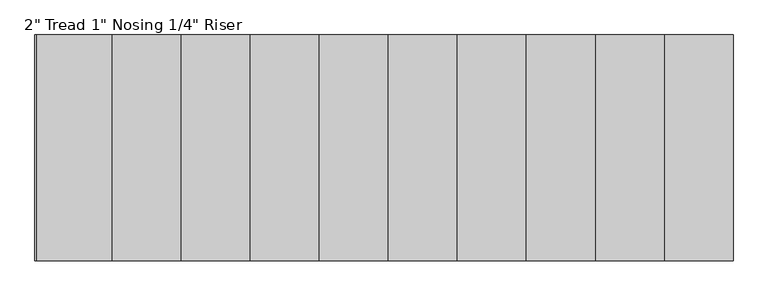
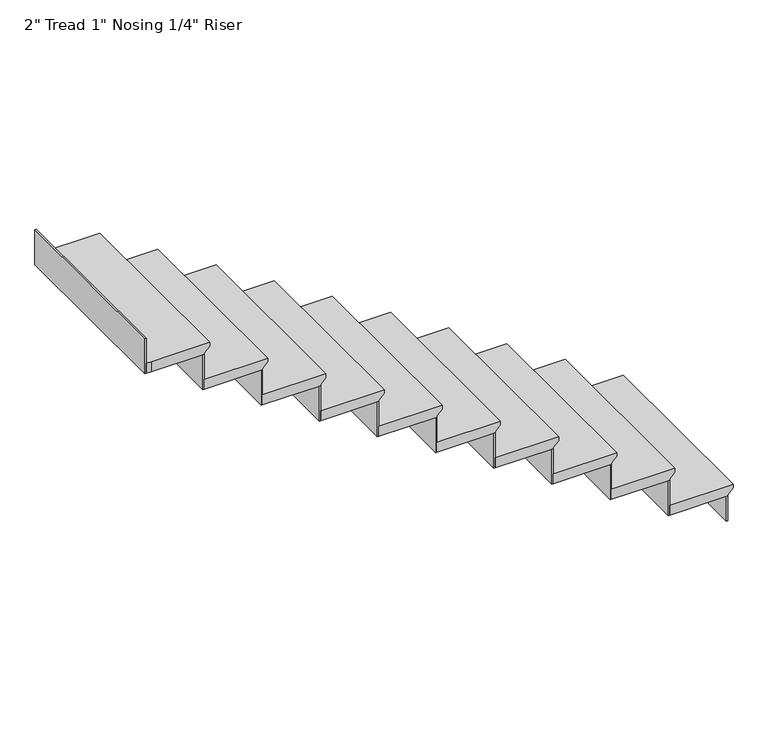
"""IFC4 building model written with IfcOpenShell, lengths in millimetres: stair flight geometry."""

from ifc_helpers import new_model, si_unit, origin, place, context, project, spatial, faceted_brep, source, transform, mapped, element, save


def stair_flight_b5a9fedd(model_context):
    return source(origin(), model_context, "Body", "Brep", [
        faceted_brep([(13347.9752377, 21801.2384539, 158.75), (13347.9752377, 21801.2384539, 177.8), (13347.9752377, 20886.8384539, 177.8), (13347.9752377, 20886.8384539, 158.75), (13322.5752377, 21801.2384539, 133.35), (13322.5752377, 20886.8384539, 133.35), (13043.1752377, 21801.2384539, 177.8), (13043.1752377, 20886.8384539, 177.8), (13322.5752377, 20886.8384539, 127.0), (13043.1752377, 20886.8384539, 127.0), (13043.1752377, 21801.2384539, 127.0), (13322.5752377, 21801.2384539, 127.0)], [[[0, 1, 2, 3]], [[4, 0, 3, 5]], [[2, 1, 6, 7]], [[8, 9, 10, 11]], [[2, 7, 9, 8, 5, 3]], [[8, 11, 4, 5]], [[6, 1, 0, 4, 11, 10]], [[7, 6, 10, 9]]]),
        faceted_brep([(13322.5752377, 21801.2384539, 127.0), (13322.5752377, 21801.2384539, 0.0), (13316.2252377, 21801.2384539, 0.0), (13316.2252377, 21801.2384539, 127.0), (13322.5752377, 20886.8384539, 127.0), (13316.2252377, 20886.8384539, 127.0), (13316.2252377, 20886.8384539, 0.0), (13322.5752377, 20886.8384539, 0.0)], [[[0, 1, 2, 3]], [[4, 5, 6, 7]], [[1, 0, 4, 7]], [[2, 1, 7, 6]], [[3, 2, 6, 5]], [[0, 3, 5, 4]]]),
        faceted_brep([(13043.1752377, 21801.2384539, 304.8), (13043.1752377, 21801.2384539, 127.0), (13036.8252377, 21801.2384539, 127.0), (13036.8252377, 21801.2384539, 304.8), (13043.1752377, 20886.8384539, 304.8), (13036.8252377, 20886.8384539, 304.8), (13036.8252377, 20886.8384539, 127.0), (13043.1752377, 20886.8384539, 127.0)], [[[0, 1, 2, 3]], [[4, 5, 6, 7]], [[1, 0, 4, 7]], [[2, 1, 7, 6]], [[3, 2, 6, 5]], [[0, 3, 5, 4]]]),
        faceted_brep([(13068.5752377, 20886.8384539, 355.6), (13068.5752377, 21801.2384539, 355.6), (12763.7752377, 21801.2384539, 355.6), (12763.7752377, 20886.8384539, 355.6), (13043.1752377, 20886.8384539, 304.8), (12763.7752377, 20886.8384539, 304.8), (12763.7752377, 21801.2384539, 304.8), (13043.1752377, 21801.2384539, 304.8), (13043.1752377, 20886.8384539, 311.15), (13068.5752377, 20886.8384539, 336.55), (13043.1752377, 21801.2384539, 311.15), (13068.5752377, 21801.2384539, 336.55)], [[[0, 1, 2, 3]], [[4, 5, 6, 7]], [[0, 3, 5, 4, 8, 9]], [[4, 7, 10, 8]], [[2, 1, 11, 10, 7, 6]], [[3, 2, 6, 5]], [[11, 1, 0, 9]], [[10, 11, 9, 8]]]),
        faceted_brep([(12763.7752377, 21801.2384539, 482.6), (12763.7752377, 21801.2384539, 304.8), (12757.4252377, 21801.2384539, 304.8), (12757.4252377, 21801.2384539, 482.6), (12763.7752377, 20886.8384539, 482.6), (12757.4252377, 20886.8384539, 482.6), (12757.4252377, 20886.8384539, 304.8), (12763.7752377, 20886.8384539, 304.8)], [[[0, 1, 2, 3]], [[4, 5, 6, 7]], [[1, 0, 4, 7]], [[2, 1, 7, 6]], [[3, 2, 6, 5]], [[0, 3, 5, 4]]]),
        faceted_brep([(12789.1752377, 20886.8384539, 533.4), (12789.1752377, 21801.2384539, 533.4), (12484.3752377, 21801.2384539, 533.4), (12484.3752377, 20886.8384539, 533.4), (12763.7752377, 20886.8384539, 482.6), (12484.3752377, 20886.8384539, 482.6), (12484.3752377, 21801.2384539, 482.6), (12763.7752377, 21801.2384539, 482.6), (12763.7752377, 20886.8384539, 488.95), (12789.1752377, 20886.8384539, 514.35), (12763.7752377, 21801.2384539, 488.95), (12789.1752377, 21801.2384539, 514.35)], [[[0, 1, 2, 3]], [[4, 5, 6, 7]], [[0, 3, 5, 4, 8, 9]], [[4, 7, 10, 8]], [[2, 1, 11, 10, 7, 6]], [[3, 2, 6, 5]], [[11, 1, 0, 9]], [[10, 11, 9, 8]]]),
        faceted_brep([(12484.3752377, 21801.2384539, 660.4), (12484.3752377, 21801.2384539, 482.6), (12478.0252377, 21801.2384539, 482.6), (12478.0252377, 21801.2384539, 660.4), (12484.3752377, 20886.8384539, 660.4), (12478.0252377, 20886.8384539, 660.4), (12478.0252377, 20886.8384539, 482.6), (12484.3752377, 20886.8384539, 482.6)], [[[0, 1, 2, 3]], [[4, 5, 6, 7]], [[1, 0, 4, 7]], [[2, 1, 7, 6]], [[3, 2, 6, 5]], [[0, 3, 5, 4]]]),
        faceted_brep([(12509.7752377, 20886.8384539, 711.2), (12509.7752377, 21801.2384539, 711.2), (12204.9752377, 21801.2384539, 711.2), (12204.9752377, 20886.8384539, 711.2), (12484.3752377, 20886.8384539, 660.4), (12204.9752377, 20886.8384539, 660.4), (12204.9752377, 21801.2384539, 660.4), (12484.3752377, 21801.2384539, 660.4), (12484.3752377, 20886.8384539, 666.75), (12509.7752377, 20886.8384539, 692.15), (12484.3752377, 21801.2384539, 666.75), (12509.7752377, 21801.2384539, 692.15)], [[[0, 1, 2, 3]], [[4, 5, 6, 7]], [[0, 3, 5, 4, 8, 9]], [[4, 7, 10, 8]], [[2, 1, 11, 10, 7, 6]], [[3, 2, 6, 5]], [[11, 1, 0, 9]], [[10, 11, 9, 8]]]),
        faceted_brep([(12204.9752377, 21801.2384539, 838.2), (12204.9752377, 21801.2384539, 660.4), (12198.6252377, 21801.2384539, 660.4), (12198.6252377, 21801.2384539, 838.2), (12204.9752377, 20886.8384539, 838.2), (12198.6252377, 20886.8384539, 838.2), (12198.6252377, 20886.8384539, 660.4), (12204.9752377, 20886.8384539, 660.4)], [[[0, 1, 2, 3]], [[4, 5, 6, 7]], [[1, 0, 4, 7]], [[2, 1, 7, 6]], [[3, 2, 6, 5]], [[0, 3, 5, 4]]]),
        faceted_brep([(12230.3752377, 20886.8384539, 889.0), (12230.3752377, 21801.2384539, 889.0), (11925.5752377, 21801.2384539, 889.0), (11925.5752377, 20886.8384539, 889.0), (12204.9752377, 20886.8384539, 838.2), (11925.5752377, 20886.8384539, 838.2), (11925.5752377, 21801.2384539, 838.2), (12204.9752377, 21801.2384539, 838.2), (12204.9752377, 20886.8384539, 844.55), (12230.3752377, 20886.8384539, 869.95), (12204.9752377, 21801.2384539, 844.55), (12230.3752377, 21801.2384539, 869.95)], [[[0, 1, 2, 3]], [[4, 5, 6, 7]], [[0, 3, 5, 4, 8, 9]], [[4, 7, 10, 8]], [[2, 1, 11, 10, 7, 6]], [[3, 2, 6, 5]], [[11, 1, 0, 9]], [[10, 11, 9, 8]]]),
        faceted_brep([(11925.5752377, 21801.2384539, 1016.0), (11925.5752377, 21801.2384539, 838.2), (11919.2252377, 21801.2384539, 838.2), (11919.2252377, 21801.2384539, 1016.0), (11925.5752377, 20886.8384539, 1016.0), (11919.2252377, 20886.8384539, 1016.0), (11919.2252377, 20886.8384539, 838.2), (11925.5752377, 20886.8384539, 838.2)], [[[0, 1, 2, 3]], [[4, 5, 6, 7]], [[1, 0, 4, 7]], [[2, 1, 7, 6]], [[3, 2, 6, 5]], [[0, 3, 5, 4]]]),
        faceted_brep([(11950.9752377, 20886.8384539, 1066.8), (11950.9752377, 21801.2384539, 1066.8), (11646.1752377, 21801.2384539, 1066.8), (11646.1752377, 20886.8384539, 1066.8), (11925.5752377, 20886.8384539, 1016.0), (11646.1752377, 20886.8384539, 1016.0), (11646.1752377, 21801.2384539, 1016.0), (11925.5752377, 21801.2384539, 1016.0), (11925.5752377, 20886.8384539, 1022.35), (11950.9752377, 20886.8384539, 1047.75), (11925.5752377, 21801.2384539, 1022.35), (11950.9752377, 21801.2384539, 1047.75)], [[[0, 1, 2, 3]], [[4, 5, 6, 7]], [[0, 3, 5, 4, 8, 9]], [[4, 7, 10, 8]], [[2, 1, 11, 10, 7, 6]], [[3, 2, 6, 5]], [[11, 1, 0, 9]], [[10, 11, 9, 8]]]),
        faceted_brep([(11646.1752377, 21801.2384539, 1193.8), (11646.1752377, 21801.2384539, 1016.0), (11639.8252377, 21801.2384539, 1016.0), (11639.8252377, 21801.2384539, 1193.8), (11646.1752377, 20886.8384539, 1193.8), (11639.8252377, 20886.8384539, 1193.8), (11639.8252377, 20886.8384539, 1016.0), (11646.1752377, 20886.8384539, 1016.0)], [[[0, 1, 2, 3]], [[4, 5, 6, 7]], [[1, 0, 4, 7]], [[2, 1, 7, 6]], [[3, 2, 6, 5]], [[0, 3, 5, 4]]]),
        faceted_brep([(11671.5752377, 20886.8384539, 1244.6), (11671.5752377, 21801.2384539, 1244.6), (11366.7752377, 21801.2384539, 1244.6), (11366.7752377, 20886.8384539, 1244.6), (11646.1752377, 20886.8384539, 1193.8), (11366.7752377, 20886.8384539, 1193.8), (11366.7752377, 21801.2384539, 1193.8), (11646.1752377, 21801.2384539, 1193.8), (11646.1752377, 20886.8384539, 1200.15), (11671.5752377, 20886.8384539, 1225.55), (11646.1752377, 21801.2384539, 1200.15), (11671.5752377, 21801.2384539, 1225.55)], [[[0, 1, 2, 3]], [[4, 5, 6, 7]], [[0, 3, 5, 4, 8, 9]], [[4, 7, 10, 8]], [[2, 1, 11, 10, 7, 6]], [[3, 2, 6, 5]], [[11, 1, 0, 9]], [[10, 11, 9, 8]]]),
        faceted_brep([(11366.7752377, 21801.2384539, 1371.6), (11366.7752377, 21801.2384539, 1193.8), (11360.4252377, 21801.2384539, 1193.8), (11360.4252377, 21801.2384539, 1371.6), (11366.7752377, 20886.8384539, 1371.6), (11360.4252377, 20886.8384539, 1371.6), (11360.4252377, 20886.8384539, 1193.8), (11366.7752377, 20886.8384539, 1193.8)], [[[0, 1, 2, 3]], [[4, 5, 6, 7]], [[1, 0, 4, 7]], [[2, 1, 7, 6]], [[3, 2, 6, 5]], [[0, 3, 5, 4]]]),
        faceted_brep([(11392.1752377, 20886.8384539, 1422.4), (11392.1752377, 21801.2384539, 1422.4), (11087.3752377, 21801.2384539, 1422.4), (11087.3752377, 20886.8384539, 1422.4), (11366.7752377, 20886.8384539, 1371.6), (11087.3752377, 20886.8384539, 1371.6), (11087.3752377, 21801.2384539, 1371.6), (11366.7752377, 21801.2384539, 1371.6), (11366.7752377, 20886.8384539, 1377.95), (11392.1752377, 20886.8384539, 1403.35), (11366.7752377, 21801.2384539, 1377.95), (11392.1752377, 21801.2384539, 1403.35)], [[[0, 1, 2, 3]], [[4, 5, 6, 7]], [[0, 3, 5, 4, 8, 9]], [[4, 7, 10, 8]], [[2, 1, 11, 10, 7, 6]], [[3, 2, 6, 5]], [[11, 1, 0, 9]], [[10, 11, 9, 8]]]),
        faceted_brep([(11087.3752377, 21801.2384539, 1549.4), (11087.3752377, 21801.2384539, 1371.6), (11081.0252377, 21801.2384539, 1371.6), (11081.0252377, 21801.2384539, 1549.4), (11087.3752377, 20886.8384539, 1549.4), (11081.0252377, 20886.8384539, 1549.4), (11081.0252377, 20886.8384539, 1371.6), (11087.3752377, 20886.8384539, 1371.6)], [[[0, 1, 2, 3]], [[4, 5, 6, 7]], [[1, 0, 4, 7]], [[2, 1, 7, 6]], [[3, 2, 6, 5]], [[0, 3, 5, 4]]]),
        faceted_brep([(11112.7752377, 20886.8384539, 1600.2), (11112.7752377, 21801.2384539, 1600.2), (10807.9752377, 21801.2384539, 1600.2), (10807.9752377, 20886.8384539, 1600.2), (11087.3752377, 20886.8384539, 1549.4), (10807.9752377, 20886.8384539, 1549.4), (10807.9752377, 21801.2384539, 1549.4), (11087.3752377, 21801.2384539, 1549.4), (11087.3752377, 20886.8384539, 1555.75), (11112.7752377, 20886.8384539, 1581.15), (11087.3752377, 21801.2384539, 1555.75), (11112.7752377, 21801.2384539, 1581.15)], [[[0, 1, 2, 3]], [[4, 5, 6, 7]], [[0, 3, 5, 4, 8, 9]], [[4, 7, 10, 8]], [[2, 1, 11, 10, 7, 6]], [[3, 2, 6, 5]], [[11, 1, 0, 9]], [[10, 11, 9, 8]]]),
        faceted_brep([(10528.5752377, 21801.2384539, 1905.0), (10528.5752377, 21801.2384539, 1727.2), (10522.2252377, 21801.2384539, 1727.2), (10522.2252377, 21801.2384539, 1905.0), (10528.5752377, 20886.8384539, 1905.0), (10522.2252377, 20886.8384539, 1905.0), (10522.2252377, 20886.8384539, 1727.2), (10528.5752377, 20886.8384539, 1727.2)], [[[0, 1, 2, 3]], [[4, 5, 6, 7]], [[1, 0, 4, 7]], [[2, 1, 7, 6]], [[3, 2, 6, 5]], [[0, 3, 5, 4]]]),
        faceted_brep([(10807.9752377, 21801.2384539, 1727.2), (10807.9752377, 21801.2384539, 1549.4), (10801.6252377, 21801.2384539, 1549.4), (10801.6252377, 21801.2384539, 1727.2), (10807.9752377, 20886.8384539, 1727.2), (10801.6252377, 20886.8384539, 1727.2), (10801.6252377, 20886.8384539, 1549.4), (10807.9752377, 20886.8384539, 1549.4)], [[[0, 1, 2, 3]], [[4, 5, 6, 7]], [[1, 0, 4, 7]], [[2, 1, 7, 6]], [[3, 2, 6, 5]], [[0, 3, 5, 4]]]),
        faceted_brep([(10528.5752377, 20886.8384539, 1778.0), (10553.9752377, 20886.8384539, 1778.0), (10833.3752377, 20886.8384539, 1778.0), (10833.3752377, 21801.2384539, 1778.0), (10528.5752377, 21801.2384539, 1778.0), (10553.9752377, 20886.8384539, 1727.2), (10528.5752377, 20886.8384539, 1727.2), (10528.5752377, 21801.2384539, 1727.2), (10807.9752377, 21801.2384539, 1727.2), (10807.9752377, 20886.8384539, 1727.2), (10807.9752377, 20886.8384539, 1733.55), (10833.3752377, 20886.8384539, 1758.95), (10807.9752377, 21801.2384539, 1733.55), (10833.3752377, 21801.2384539, 1758.95)], [[[0, 1, 2, 3, 4]], [[5, 6, 7, 8, 9]], [[1, 0, 6, 5]], [[2, 1, 5, 9, 10, 11]], [[9, 8, 12, 10]], [[4, 3, 13, 12, 8, 7]], [[0, 4, 7, 6]], [[13, 3, 2, 11]], [[12, 13, 11, 10]]]),
    ])


if __name__ == "__main__":
    model = new_model("IFC4")
    model_context = context("Model", 3, world=origin())
    ifc_project = project(units=[si_unit("LENGTHUNIT", "METRE", prefix="MILLI")], contexts=[model_context])
    site = spatial("IfcSite", under=ifc_project)
    building = spatial("IfcBuilding", under=site)
    placement = place(None, origin())
    stair_flight_shape = stair_flight_b5a9fedd(model_context)
    element("IfcStairFlight", 1, ObjectType="2\" Tread 1\" Nosing 1/4\" Riser", at=placement, inside=building, context=model_context, shape_type="MappedRepresentation", body=[
        mapped(stair_flight_shape, transform((0.0, 0.0, 0.0), x_axis=(1.0, 0.0, 0.0), y_axis=(0.0, 1.0, 0.0), z_axis=(0.0, 0.0, 1.0))),
    ])
    save(model, "model.ifc")
